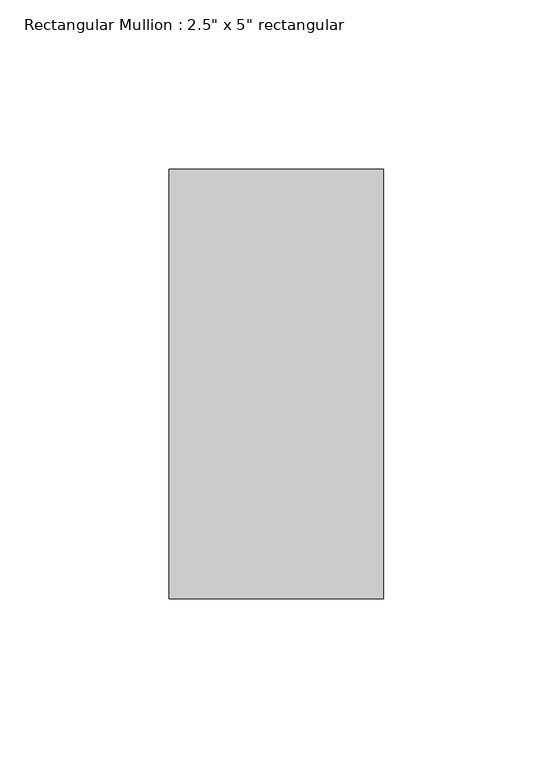
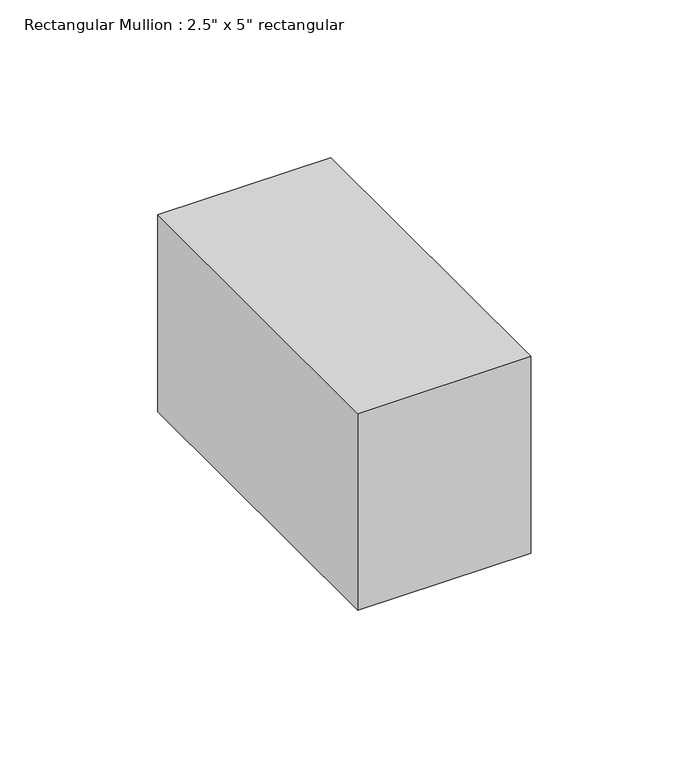
"""IFC4 building model written with IfcOpenShell, lengths in millimetres: member geometry."""

from ifc_helpers import new_model, si_unit, frame, origin, place, context, project, spatial, polyline, outline, extrude, source, transform, mapped, element, save


def member_00d00b53(model_context):
    return source(origin(), model_context, "Body", "SweptSolid", [
        extrude(outline(polyline([(31.75, 63.5), (31.75, -63.5), (-31.75, -63.5), (-31.75, 63.5), (31.75, 63.5)])), frame((0.0, 0.0, -76.2), z_axis=(0.0, 0.0, 1.0), x_axis=(1.0, 0.0, 0.0)), (0.0, 0.0, 1.0), 76.2),
    ])


if __name__ == "__main__":
    model = new_model("IFC4")
    model_context = context("Model", 3, world=origin())
    ifc_project = project(units=[si_unit("LENGTHUNIT", "METRE", prefix="MILLI")], contexts=[model_context])
    site = spatial("IfcSite", under=ifc_project)
    building = spatial("IfcBuilding", under=site)
    placement = place(None, origin())
    member_shape = member_00d00b53(model_context)
    element("IfcMember", 1, ObjectType="Rectangular Mullion : 2.5\" x 5\" rectangular", at=placement, inside=building, context=model_context, shape_type="MappedRepresentation", body=[
        mapped(member_shape, transform((0.0, 0.0, 0.0), x_axis=(1.0, 0.0, 0.0), y_axis=(0.0, 1.0, 0.0), z_axis=(0.0, 0.0, 1.0))),
    ])
    save(model, "model.ifc")

# Revit data of these elements
# Type "Rectangular Mullion : 2.5\" x 5\" rectangular"
#   built-in parameter 1007304 = 0.416667 (stored number, unit not read)
#   built-in parameter 1007301 = 0.104167 (stored number, unit not read)
#   built-in parameter 1007300 = 0.104167 (stored number, unit not read)
# Element 1 (IfcMember, "Rectangular Mullion : 2.5\" x 5\" rectangular")
#   Materials on its faces: "Aluminum"
# Materials
#   "Aluminum": class "Metal", colour RGB 247 247 247, transparency 0, Description = "Aluminum 6061", Cost = 0
